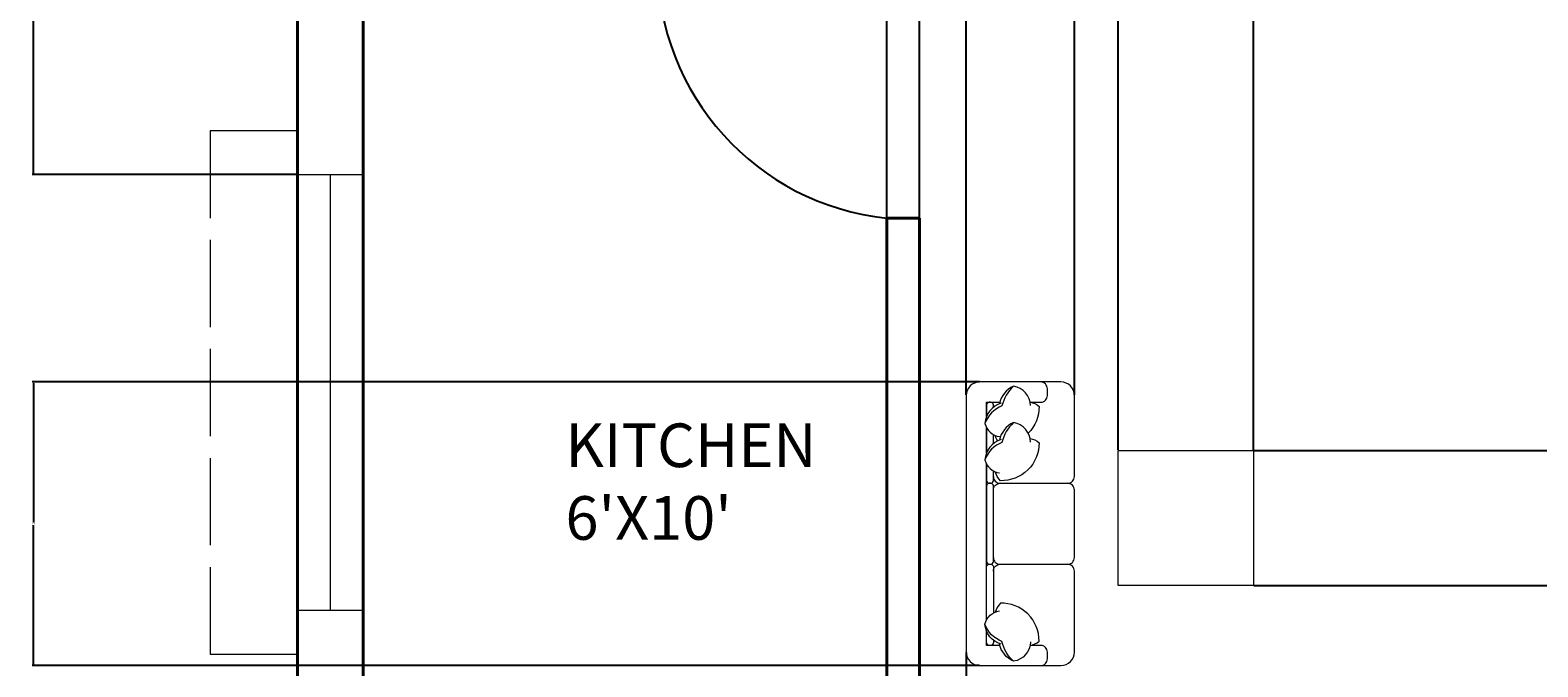
# Model space of a CAD drawing. Units: inches. Extents: x -22 to 362, y -469 to 42.
# Tile 2 of 6: x -22 to 186, y -295 to -207. Entities that reach past the tile are written whole.
import ezdxf

# ---------------------------------------------------------------- set-up
doc = ezdxf.new("R2010")
doc.units = ezdxf.units.IN
doc.header["$MEASUREMENT"] = 0
doc.linetypes.add('ACAD_ISO02W100', pattern=[15, 12, -3])
for name, color, linetype, lineweight in [('A-ANNO-DIMS', 2, 'Continuous', 18), ('A-AREA-IDEN', 7, 'Continuous', 25), ('A-DOOR', 3, 'Continuous', 25), ('A-FURN', 8, 'Continuous', 18), ('A-GLAZ', 4, 'Continuous', 20), ('A-ROOF-OVHD', 8, 'ACAD_ISO02W100', 18), ('A-WALL', 7, 'Continuous', 40)]:
    doc.layers.add(name, color=color, linetype=linetype, lineweight=lineweight)
doc.styles.get("Standard").update_dxf_attribs({"font": 'arial.ttf'})
doc.dimstyles.get("Standard").update_dxf_attribs({"dimtxt": 0.18, "dimasz": 0.18, "dimexe": 0.18, "dimexo": 0.0625, "dimgap": 0.09, "dimtad": 0, "dimtih": 1, "dimtoh": 1, "dimdec": 0, "dimzin": 0, "dimdsep": 46, "dimlunit": 3, "dimtxsty": 'Standard', "dimcen": 0.09, "dimadec": 0, "dimazin": 0, "dimtfac": 1, "dimtdec": 0, "dimtofl": 0, "dimtmove": 0, "dimatfit": 3, "dimfxl": 1, "dimtolj": 1, "dimtzin": 0, "dimarcsym": 0})

# ---------------------------------------------------------------- blocks, each defined once
blk = doc.blocks.new('DOOR-SWING-36')
for p, q in [((-1, 0), (-1, 36)), ((0, 0), (-1, 0))]:
    blk.add_line(p, q)
blk.add_arc((-1, 0.81), 35.19, 90, 173.9744)
blk = doc.blocks.new('WIN-60-WALL9')
for p, q in [((0, 9), (60, 9)), ((0, 0), (0, 9)), ((60, 9), (60, 0)), ((0, 4.5), (60, 4.5)), ((60, 0), (0, 0))]:
    blk.add_line(p, q)
blk = doc.blocks.new('WINDOW-SHADE-72')
for p, q in [((12, 72), (0, 72)), ((12, 0), (12, 72)), ((0, 0), (12, 0))]:
    blk.add_line(p, q)
blk = doc.blocks.new('*D36')
at = {"layer": 'A-ANNO-DIMS', "color": 0, "lineweight": -2, "transparency": 16777216}
for p, q in [((14.95, -176.52), (-21.45, -176.52)), ((-21.27, -176.7), (-21.27, -201.48)), ((-21.27, -226.63), (-21.27, -201.85)), ((14.95, -226.81), (-21.45, -226.81))]:
    blk.add_line(p, q, dxfattribs=at)
at = {"layer": 'A-ANNO-DIMS', "color": 0, "transparency": 16777216}
for points in [[(-21.3, -176.7), (-21.24, -176.7), (-21.27, -176.52)], [(-21.3, -226.63), (-21.24, -226.63), (-21.27, -226.81)]]:
    blk.add_solid(points, dxfattribs=at)
at = {"layer": 'Defpoints', "color": 0, "transparency": 16777216}
for p in [(15.01, -176.52), (-21.27, -226.81), (15.01, -226.81)]:
    blk.add_point(p, dxfattribs=at)
at = {"layer": 'A-ANNO-DIMS', "color": 0, "transparency": 16777216, "insert": (-21.27, -201.66), "char_height": 0.18, "attachment_point": 5}
blk.add_mtext('\\A1;4\'-2 1/2"', dxfattribs=at)
blk = doc.blocks.new('*D51')
at = {"layer": 'A-ANNO-DIMS', "color": 0, "lineweight": -2, "transparency": 16777216}
for p, q in [((96.01, -232.74), (96.01, 42.15)), ((96.19, 41.97), (97.72, 41.97)), ((100.33, 41.97), (98.8, 41.97)), ((100.51, -232.74), (100.51, 42.15))]:
    blk.add_line(p, q, dxfattribs=at)
at = {"layer": 'A-ANNO-DIMS', "color": 0, "transparency": 16777216}
for points in [[(96.19, 42), (96.19, 41.94), (96.01, 41.97)], [(100.33, 42), (100.33, 41.94), (100.51, 41.97)]]:
    blk.add_solid(points, dxfattribs=at)
at = {"layer": 'Defpoints', "color": 0, "transparency": 16777216}
for p in [(100.51, 41.97), (96.01, -232.81), (100.51, -232.81)]:
    blk.add_point(p, dxfattribs=at)
at = {"layer": 'A-ANNO-DIMS', "color": 0, "transparency": 16777216, "insert": (98.26, 41.97), "char_height": 0.18, "attachment_point": 5}
blk.add_mtext('\\A1;0\'-4 1/2"', dxfattribs=at)
blk = doc.blocks.new('*D52')
at = {"layer": 'A-ANNO-DIMS', "color": 0, "lineweight": -2, "transparency": 16777216}
for p, q in [((106.94, -292.58), (106.94, -468.77)), ((100.51, -316.87), (100.51, -468.77)), ((100.69, -468.59), (103.19, -468.59)), ((106.76, -468.59), (104.27, -468.59))]:
    blk.add_line(p, q, dxfattribs=at)
at = {"layer": 'A-ANNO-DIMS', "color": 0, "transparency": 16777216}
for points in [[(100.69, -468.56), (100.69, -468.62), (100.51, -468.59)], [(106.76, -468.56), (106.76, -468.62), (106.94, -468.59)]]:
    blk.add_solid(points, dxfattribs=at)
at = {"layer": 'Defpoints', "color": 0, "transparency": 16777216}
for p in [(106.94, -292.52), (100.51, -316.81), (106.94, -468.59)]:
    blk.add_point(p, dxfattribs=at)
at = {"layer": 'A-ANNO-DIMS', "color": 0, "transparency": 16777216, "insert": (103.73, -468.59), "char_height": 0.18, "attachment_point": 5}
blk.add_mtext('\\A1;0\'-6 1/2"', dxfattribs=at)
blk = doc.blocks.new('*D54')
at = {"layer": 'A-ANNO-DIMS', "color": 0, "lineweight": -2, "transparency": 16777216}
for p, q in [((108.74, -255.35), (-21.45, -255.35)), ((-21.27, -255.53), (-21.27, -274.68)), ((-21.27, -294.19), (-21.27, -275.04)), ((108.74, -294.37), (-21.45, -294.37))]:
    blk.add_line(p, q, dxfattribs=at)
at = {"layer": 'A-ANNO-DIMS', "color": 0, "transparency": 16777216}
for points in [[(-21.3, -255.53), (-21.24, -255.53), (-21.27, -255.35)], [(-21.3, -294.19), (-21.24, -294.19), (-21.27, -294.37)]]:
    blk.add_solid(points, dxfattribs=at)
at = {"layer": 'Defpoints', "color": 0, "transparency": 16777216}
for p in [(108.8, -255.35), (-21.27, -294.37), (108.8, -294.37)]:
    blk.add_point(p, dxfattribs=at)
at = {"layer": 'A-ANNO-DIMS', "color": 0, "transparency": 16777216, "insert": (-21.27, -274.86), "char_height": 0.18, "attachment_point": 5}
blk.add_mtext('\\A1;3\'-3"', dxfattribs=at)
blk = doc.blocks.new('*D55')
at = {"layer": 'A-ANNO-DIMS', "color": 0, "lineweight": -2, "transparency": 16777216}
for p, q in [((106.94, -257.14), (106.94, 42.15)), ((107.12, 41.97), (114.06, 41.97)), ((121.63, 41.97), (114.7, 41.97)), ((121.81, -257.14), (121.81, 42.15))]:
    blk.add_line(p, q, dxfattribs=at)
at = {"layer": 'A-ANNO-DIMS', "color": 0, "transparency": 16777216}
for points in [[(107.12, 42), (107.12, 41.94), (106.94, 41.97)], [(121.63, 42), (121.63, 41.94), (121.81, 41.97)]]:
    blk.add_solid(points, dxfattribs=at)
at = {"layer": 'Defpoints', "color": 0, "transparency": 16777216}
for p in [(121.81, 41.97), (106.94, -257.21), (121.81, -257.21)]:
    blk.add_point(p, dxfattribs=at)
at = {"layer": 'A-ANNO-DIMS', "color": 0, "transparency": 16777216, "insert": (114.38, 41.97), "char_height": 0.18, "attachment_point": 5}
blk.add_mtext('\\A1;1\'-3"', dxfattribs=at)
blk = doc.blocks.new('*D56')
at = {"layer": 'A-ANNO-DIMS', "color": 0, "lineweight": -2, "transparency": 16777216}
for p, q in [((127.83, -264.69), (127.83, 42.15)), ((128.01, 41.97), (136.59, 41.97)), ((146.23, 41.97), (137.65, 41.97)), ((146.41, -264.69), (146.41, 42.15))]:
    blk.add_line(p, q, dxfattribs=at)
at = {"layer": 'A-ANNO-DIMS', "color": 0, "transparency": 16777216}
for points in [[(128.01, 42), (128.01, 41.94), (127.83, 41.97)], [(146.23, 42), (146.23, 41.94), (146.41, 41.97)]]:
    blk.add_solid(points, dxfattribs=at)
at = {"layer": 'Defpoints', "color": 0, "transparency": 16777216}
for p in [(146.41, 41.97), (127.83, -264.76), (146.41, -264.76)]:
    blk.add_point(p, dxfattribs=at)
at = {"layer": 'A-ANNO-DIMS', "color": 0, "transparency": 16777216, "insert": (137.12, 41.97), "char_height": 0.18, "attachment_point": 5}
blk.add_mtext('\\A1;1\'-6 1/2"', dxfattribs=at)
blk = doc.blocks.new('*D57')
at = {"layer": 'A-ANNO-DIMS', "color": 0, "lineweight": -2, "transparency": 16777216}
for p, q in [((146.47, -264.76), (350.97, -264.76)), ((350.79, -264.94), (350.79, -273.87)), ((350.79, -283.16), (350.79, -274.23)), ((146.47, -283.34), (350.97, -283.34))]:
    blk.add_line(p, q, dxfattribs=at)
at = {"layer": 'A-ANNO-DIMS', "color": 0, "transparency": 16777216}
for points in [[(350.76, -264.94), (350.82, -264.94), (350.79, -264.76)], [(350.76, -283.16), (350.82, -283.16), (350.79, -283.34)]]:
    blk.add_solid(points, dxfattribs=at)
at = {"layer": 'Defpoints', "color": 0, "transparency": 16777216}
for p in [(146.41, -264.76), (146.41, -283.34), (350.79, -283.34)]:
    blk.add_point(p, dxfattribs=at)
at = {"layer": 'A-ANNO-DIMS', "color": 0, "transparency": 16777216, "insert": (350.79, -274.05), "char_height": 0.18, "attachment_point": 5}
blk.add_mtext('\\A1;1\'-6 1/2"', dxfattribs=at)

msp = doc.modelspace()

# ---------------------------------------------------------------- linework, layer by layer
at = {"layer": 'A-FURN', "ltscale": 0.03}
msp.add_lwpolyline([(119.95, -294.37, 0.414214), (121.81, -292.52), (121.81, -281.36, 0.414214), (120.88, -280.44, 0.414214), (121.81, -279.51), (121.81, -270.21, 0.414214), (120.88, -269.29, 0.414214), (121.81, -268.36), (121.81, -257.21, 0.414214), (119.95, -255.35), (108.8, -255.35, 0.414214), (106.94, -257.21), (106.94, -292.52, 0.414214), (108.8, -294.37)], format="xyb", close=True, dxfattribs=at)
at = {"layer": 'A-FURN'}
for points in [[(113.44, -255.94, 0.14773), (111.84, -258.65, 0.213343), (109.5, -261.05, 0.178662)], [(115.78, -258.6, 0.356772), (113.44, -255.94, 0.249542), (111.51, -258.35, -9.61688)], [(115.73, -258.13), (117.17, -258.13, 0.414214), (118.09, -257.21), (118.09, -256.28, 0.414214), (117.17, -255.35)], [(111.72, -258.28, 0.306663), (109.5, -261.05, 0.30633), (111.52, -262.86, -0.872847)], [(109.73, -260.09), (109.73, -258.13), (111.56, -258.13, 0.414214)], [(110.66, -258.84), (110.66, -258.51, 0.414214), (110.29, -258.13), (110.1, -258.13, 0.414214), (109.73, -258.51)], [(109.73, -258.51), (109.73, -260.09, 0.414214)], [(115.72, -258.13, -0.165541), (116.95, -258.71, -0.200231), (115.46, -262.4, -0.121523)], [(113.44, -260.94, 0.14773), (111.84, -263.66, 0.213343), (109.5, -266.06, 0.178662)], [(115.78, -263.61, 0.356772), (113.44, -260.94, 0.249542), (111.51, -263.36, -9.61688)], [(109.73, -261.64), (109.73, -265.09, 0.414214)], [(110.66, -263.85), (110.66, -262.57, 0.414214)], [(111.26, -263.47, -0.071865), (110.9, -262.69, 7.115464)], [(115.72, -263.14, -0.165541), (116.95, -263.71, -0.425989), (111.63, -268.93, -0.121523), (110.9, -267.69, 7.115464)], [(111.72, -263.28, 0.306663), (109.5, -266.06, 0.30633), (111.52, -267.87, -0.872847)], [(109.73, -266.64), (109.73, -268.91, 0.414214), (110.1, -269.29), (110.29, -269.29, 0.414214), (110.66, -268.91), (110.66, -267.58, 0.414214)], [(110.66, -268.36, 0.414214), (111.59, -269.29), (120.88, -269.29, 0.414214)], [(110.66, -270.21, -0.414214), (111.59, -269.29)], [(110.66, -279.51, 0.414214), (111.59, -280.44)], [(109.73, -288.09), (109.73, -280.81, -0.414214), (110.1, -280.44), (110.29, -280.44, -0.414214), (110.66, -280.81), (110.66, -287.15, -0.414214)], [(110.66, -281.36, -0.414214), (111.59, -280.44), (120.88, -280.44, -0.414214)], [(115.72, -291.59, 0.165541), (116.95, -291.01, 0.425989), (111.63, -285.79, 0.121523), (110.9, -287.03, -7.115464)], [(111.72, -291.44, -0.306663), (109.5, -288.67, -0.30633), (111.52, -286.86, 0.872847)], [(113.44, -293.78, -0.14773), (111.84, -291.07, -0.213343), (109.5, -288.67, -0.178662)], [(109.73, -291.21), (109.73, -289.63, -0.414214)], [(110.66, -290.88), (110.66, -291.21, -0.414214), (110.29, -291.59), (110.1, -291.59, -0.414214), (109.73, -291.21)], [(115.78, -291.12, -0.356772), (113.44, -293.78, -0.249542), (111.51, -291.37, 9.61688)], [(117.17, -294.37, 0.414214), (118.09, -293.44), (118.09, -292.52, 0.414214), (117.17, -291.59), (115.73, -291.59)]]:
    msp.add_lwpolyline(points, format="xyb", dxfattribs=at)
for points in [[(109.73, -265.09), (109.73, -261.64)], [(109.73, -288.09), (109.73, -266.64)], [(111.56, -291.59), (109.73, -291.59), (109.73, -289.63)]]:
    msp.add_lwpolyline(points, dxfattribs=at)
at = {"layer": 'A-FURN', "ltscale": 0.03}
msp.add_lwpolyline([(146.41, -264.76), (146.41, -283.34), (127.83, -283.34), (127.83, -264.76)], close=True, dxfattribs=at)
at = {"layer": 'A-FURN'}
msp.add_lwpolyline([(109.73, -269.66), (109.73, -280.06, 0.414214), (110.1, -280.44), (110.29, -280.44, 0.414214), (110.66, -280.06), (110.66, -269.66, 0.414214), (110.29, -269.29), (110.1, -269.29, 0.414214)], format="xyb", close=True, dxfattribs=at)
at = {"layer": 'A-WALL'}
for p, q in [((15.01, 5.69), (15.01, -414.31)), ((24.01, -196.81), (24.01, -316.81)), ((96.01, -232.81), (96.01, -316.81)), ((100.51, -232.81), (96.01, -232.81)), ((100.51, -232.81), (100.51, -316.81))]:
    msp.add_line(p, q, dxfattribs=at)

# ---------------------------------------------------------------- block references
at = {"layer": 'A-DOOR', "rotation": 90}
msp.add_blockref('DOOR-SWING-36', (100.51, -196.81), dxfattribs=at)
at = {"layer": 'A-GLAZ', "rotation": 270}
msp.add_blockref('WIN-60-WALL9', (15.01, -226.81), dxfattribs=at)
at = {"layer": 'A-ROOF-OVHD', "rotation": 180}
msp.add_blockref('WINDOW-SHADE-72', (15.01, -220.81), dxfattribs=at)

# ---------------------------------------------------------------- texts
at = {"layer": 'A-AREA-IDEN', "insert": (51.84, -261.06), "char_height": 6, "attachment_point": 1}
msp.add_mtext("KITCHEN\\P6'X10'", dxfattribs=at)

# ---------------------------------------------------------------- dimensions: what is measured, and where the dimension line sits
at = {"layer": 'A-ANNO-DIMS'}
for base, p1, p2, picture, middle in [((100.51, 41.97), (96.01, -232.81), (100.51, -232.81), '*D51', (98.26, 41.97)), ((121.81, 41.97), (106.94, -257.21), (121.81, -257.21), '*D55', (114.38, 41.97)), ((146.41, 41.97), (127.83, -264.76), (146.41, -264.76), '*D56', (137.12, 41.97)), ((106.94, -468.59), (100.51, -316.81), (106.94, -292.52), '*D52', (103.73, -468.59))]:
    dim = msp.add_linear_dim(base=base, p1=p1, p2=p2, dimstyle='Standard', override={"dimdec": 1, "dimlfac": 1, "dimrnd": 0, "dimzin": 1, "dimdsep": 46, "dimlunit": 4, "dimfrac": 2}, dxfattribs=at)
    dim.commit()
    dim.dimension.update_dxf_attribs({"geometry": picture, "text_midpoint": middle})
for base, p1, p2, picture, middle in [((-21.27, -226.81), (15.01, -176.52), (15.01, -226.81), '*D36', (-21.27, -201.66)), ((-21.27, -294.37), (108.8, -255.35), (108.8, -294.37), '*D54', (-21.27, -274.86)), ((350.79, -283.34), (146.41, -264.76), (146.41, -283.34), '*D57', (350.79, -274.05))]:
    dim = msp.add_linear_dim(base=base, p1=p1, p2=p2, angle=90, dimstyle='Standard', override={"dimdec": 1, "dimlfac": 1, "dimrnd": 0, "dimzin": 1, "dimdsep": 46, "dimlunit": 4, "dimfrac": 2}, dxfattribs=at)
    dim.commit()
    dim.dimension.update_dxf_attribs({"geometry": picture, "text_midpoint": middle})

doc.saveas('drawing.dxf')
